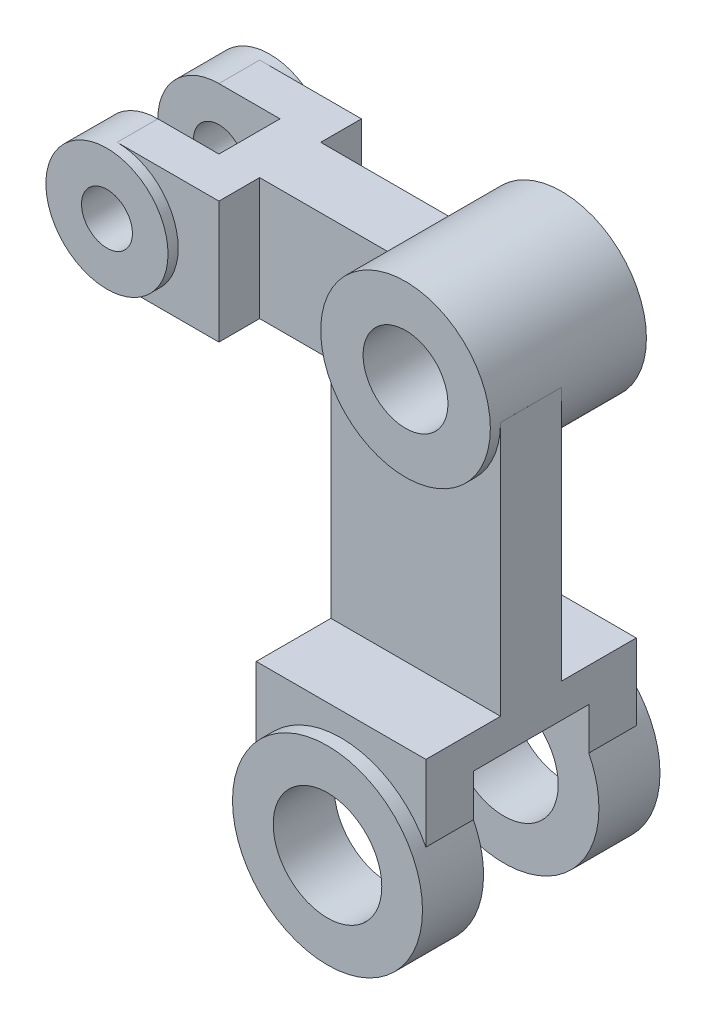
ISO-10303-21;
HEADER;
FILE_DESCRIPTION(('STEP AP214'),'2;1');
FILE_NAME('part.step','',(''),(''),'','','');
FILE_SCHEMA(('AUTOMOTIVE_DESIGN { 1 0 10303 214 1 1 1 1 }'));
ENDSEC;
DATA;
#1=APPLICATION_CONTEXT('core data for automotive mechanical design processes');
#2=APPLICATION_PROTOCOL_DEFINITION('international standard','automotive_design',2000,#1);
#3=PRODUCT_CONTEXT('',#1,'mechanical');
#4=PRODUCT('Part','Part','',(#3));
#5=PRODUCT_RELATED_PRODUCT_CATEGORY('part','',(#4));
#6=PRODUCT_DEFINITION_FORMATION('','',#4);
#7=PRODUCT_DEFINITION_CONTEXT('part definition',#1,'design');
#8=PRODUCT_DEFINITION('design','',#6,#7);
#9=PRODUCT_DEFINITION_SHAPE('','',#8);
#10=(LENGTH_UNIT() NAMED_UNIT(*) SI_UNIT(.MILLI.,.METRE.));
#11=(NAMED_UNIT(*) PLANE_ANGLE_UNIT() SI_UNIT($,.RADIAN.));
#12=(NAMED_UNIT(*) SI_UNIT($,.STERADIAN.) SOLID_ANGLE_UNIT());
#13=UNCERTAINTY_MEASURE_WITH_UNIT(LENGTH_MEASURE(1.E-05),#10,'distance_accuracy_value','');
#14=(GEOMETRIC_REPRESENTATION_CONTEXT(3) GLOBAL_UNCERTAINTY_ASSIGNED_CONTEXT((#13)) GLOBAL_UNIT_ASSIGNED_CONTEXT((#10,
#11,#12)) REPRESENTATION_CONTEXT('',''));
#15=CARTESIAN_POINT('',(0.,0.,0.));
#16=DIRECTION('',(0.,0.,1.));
#17=DIRECTION('',(1.,0.,0.));
#18=AXIS2_PLACEMENT_3D('',#15,#16,#17);
#19=CARTESIAN_POINT('',(0.,110.,0.));
#20=DIRECTION('',(0.,1.,0.));
#21=DIRECTION('',(0.,0.,1.));
#22=AXIS2_PLACEMENT_3D('',#19,#20,#21);
#23=PLANE('',#22);
#24=DIRECTION('',(1.,0.,0.));
#25=VECTOR('',#24,1.);
#26=CARTESIAN_POINT('',(0.,110.,-35.));
#27=LINE('',#26,#25);
#28=CARTESIAN_POINT('',(-25.,110.,-35.));
#29=VERTEX_POINT('',#28);
#30=CARTESIAN_POINT('',(-24.9978511346783,110.,-35.));
#31=VERTEX_POINT('',#30);
#32=EDGE_CURVE('E316',#29,#31,#27,.T.);
#33=ORIENTED_EDGE('',*,*,#32,.F.);
#34=DIRECTION('',(0.,0.,1.));
#35=VECTOR('',#34,1.);
#36=CARTESIAN_POINT('',(-25.,110.,-44.));
#37=LINE('',#36,#35);
#38=CARTESIAN_POINT('',(-25.,110.,-26.));
#39=VERTEX_POINT('',#38);
#40=EDGE_CURVE('E346',#29,#39,#37,.T.);
#41=ORIENTED_EDGE('',*,*,#40,.T.);
#42=DIRECTION('',(1.,0.,0.));
#43=VECTOR('',#42,1.);
#44=CARTESIAN_POINT('',(-25.,110.,-26.));
#45=LINE('',#44,#43);
#46=CARTESIAN_POINT('',(-24.9978511346783,110.,-26.));
#47=VERTEX_POINT('',#46);
#48=EDGE_CURVE('E351',#39,#47,#45,.T.);
#49=ORIENTED_EDGE('',*,*,#48,.T.);
#50=DIRECTION('',(0.,0.,1.));
#51=VECTOR('',#50,1.);
#52=CARTESIAN_POINT('',(-24.9978511346783,110.,-69.));
#53=LINE('',#52,#51);
#54=EDGE_CURVE('E465',#31,#47,#53,.T.);
#55=ORIENTED_EDGE('',*,*,#54,.F.);
#56=EDGE_LOOP('',(#33,#41,#49,#55));
#57=FACE_BOUND('',#56,.T.);
#58=ADVANCED_FACE('F44',(#57),#23,.T.);
#59=CARTESIAN_POINT('',(0.,35.,0.));
#60=DIRECTION('',(0.,-1.,0.));
#61=DIRECTION('',(0.,0.,-1.));
#62=AXIS2_PLACEMENT_3D('',#59,#60,#61);
#63=PLANE('',#62);
#64=DIRECTION('',(-1.,0.,0.));
#65=VECTOR('',#64,1.);
#66=CARTESIAN_POINT('',(-25.,35.,-44.));
#67=LINE('',#66,#65);
#68=CARTESIAN_POINT('',(25.0042977306435,35.,-44.));
#69=VERTEX_POINT('',#68);
#70=CARTESIAN_POINT('',(-25.,35.,-44.));
#71=VERTEX_POINT('',#70);
#72=EDGE_CURVE('E354',#69,#71,#67,.T.);
#73=ORIENTED_EDGE('',*,*,#72,.F.);
#74=DIRECTION('',(0.,0.,-1.));
#75=VECTOR('',#74,1.);
#76=CARTESIAN_POINT('',(25.0042977306435,35.,0.));
#77=LINE('',#76,#75);
#78=CARTESIAN_POINT('',(25.0042977306435,35.,-66.));
#79=VERTEX_POINT('',#78);
#80=EDGE_CURVE('E448',#69,#79,#77,.T.);
#81=ORIENTED_EDGE('',*,*,#80,.T.);
#82=DIRECTION('',(-1.,0.,0.));
#83=VECTOR('',#82,1.);
#84=CARTESIAN_POINT('',(-28.,35.,-66.));
#85=LINE('',#84,#83);
#86=CARTESIAN_POINT('',(-25.,35.,-66.));
#87=VERTEX_POINT('',#86);
#88=EDGE_CURVE('E429',#79,#87,#85,.T.);
#89=ORIENTED_EDGE('',*,*,#88,.T.);
#90=DIRECTION('',(0.,0.,1.));
#91=VECTOR('',#90,1.);
#92=CARTESIAN_POINT('',(-25.,35.,0.));
#93=LINE('',#92,#91);
#94=EDGE_CURVE('E450',#87,#71,#93,.T.);
#95=ORIENTED_EDGE('',*,*,#94,.T.);
#96=EDGE_LOOP('',(#73,#81,#89,#95));
#97=FACE_BOUND('',#96,.T.);
#98=ADVANCED_FACE('F520',(#97),#63,.F.);
#99=DIRECTION('',(1.,0.,0.));
#100=VECTOR('',#99,1.);
#101=CARTESIAN_POINT('',(-25.,35.,-26.));
#102=LINE('',#101,#100);
#103=CARTESIAN_POINT('',(-25.,35.,-26.));
#104=VERTEX_POINT('',#103);
#105=CARTESIAN_POINT('',(25.0042977306435,35.,-26.));
#106=VERTEX_POINT('',#105);
#107=EDGE_CURVE('E350',#104,#106,#102,.T.);
#108=ORIENTED_EDGE('',*,*,#107,.F.);
#109=CARTESIAN_POINT('',(-25.,35.,-4.));
#110=VERTEX_POINT('',#109);
#111=EDGE_CURVE('E447',#104,#110,#93,.T.);
#112=ORIENTED_EDGE('',*,*,#111,.T.);
#113=DIRECTION('',(1.,0.,0.));
#114=VECTOR('',#113,1.);
#115=CARTESIAN_POINT('',(28.,35.,-4.));
#116=LINE('',#115,#114);
#117=CARTESIAN_POINT('',(25.0042977306435,35.,-4.));
#118=VERTEX_POINT('',#117);
#119=EDGE_CURVE('E428',#110,#118,#116,.T.);
#120=ORIENTED_EDGE('',*,*,#119,.T.);
#121=EDGE_CURVE('E452',#118,#106,#77,.T.);
#122=ORIENTED_EDGE('',*,*,#121,.T.);
#123=EDGE_LOOP('',(#108,#112,#120,#122));
#124=FACE_BOUND('',#123,.T.);
#125=ADVANCED_FACE('F527',(#124),#63,.F.);
#126=CARTESIAN_POINT('',(0.,0.,-70.));
#127=DIRECTION('',(0.,0.,1.));
#128=DIRECTION('',(1.,0.,0.));
#129=AXIS2_PLACEMENT_3D('',#126,#127,#128);
#130=CYLINDRICAL_SURFACE('',#129,28.);
#131=CARTESIAN_POINT('',(0.,0.,-70.));
#132=DIRECTION('',(0.,0.,1.));
#133=DIRECTION('',(1.,0.,0.));
#134=AXIS2_PLACEMENT_3D('',#131,#132,#133);
#135=CIRCLE('',#134,28.);
#136=CARTESIAN_POINT('',(28.,0.,-70.));
#137=VERTEX_POINT('',#136);
#138=EDGE_CURVE('E416',#137,#137,#135,.T.);
#139=ORIENTED_EDGE('',*,*,#138,.T.);
#140=EDGE_LOOP('',(#139));
#141=FACE_BOUND('',#140,.T.);
#142=CARTESIAN_POINT('',(0.,0.,-66.));
#143=DIRECTION('',(0.,0.,-1.));
#144=DIRECTION('',(-1.,0.,0.));
#145=AXIS2_PLACEMENT_3D('',#142,#143,#144);
#146=CIRCLE('',#145,28.);
#147=CARTESIAN_POINT('',(-25.,12.6095202129185,-66.));
#148=VERTEX_POINT('',#147);
#149=CARTESIAN_POINT('',(25.0042977306435,12.6009957938782,-66.));
#150=VERTEX_POINT('',#149);
#151=EDGE_CURVE('E422',#148,#150,#146,.T.);
#152=ORIENTED_EDGE('',*,*,#151,.T.);
#153=DIRECTION('',(0.,0.,1.));
#154=VECTOR('',#153,1.);
#155=CARTESIAN_POINT('',(25.0042977306435,12.6009957938782,-70.));
#156=LINE('',#155,#154);
#157=CARTESIAN_POINT('',(25.0042977306435,12.6009957938782,-52.));
#158=VERTEX_POINT('',#157);
#159=EDGE_CURVE('E376',#150,#158,#156,.T.);
#160=ORIENTED_EDGE('',*,*,#159,.T.);
#161=CARTESIAN_POINT('',(0.,0.,-52.));
#162=DIRECTION('',(0.,0.,1.));
#163=DIRECTION('',(1.,0.,0.));
#164=AXIS2_PLACEMENT_3D('',#161,#162,#163);
#165=CIRCLE('',#164,28.);
#166=CARTESIAN_POINT('',(-25.,12.6095202129185,-52.));
#167=VERTEX_POINT('',#166);
#168=EDGE_CURVE('E417',#167,#158,#165,.T.);
#169=ORIENTED_EDGE('',*,*,#168,.F.);
#170=DIRECTION('',(0.,0.,1.));
#171=VECTOR('',#170,1.);
#172=CARTESIAN_POINT('',(-25.,12.6095202129185,-70.));
#173=LINE('',#172,#171);
#174=EDGE_CURVE('E383',#167,#148,#173,.F.);
#175=ORIENTED_EDGE('',*,*,#174,.T.);
#176=EDGE_LOOP('',(#152,#160,#169,#175));
#177=FACE_BOUND('',#176,.T.);
#178=ADVANCED_FACE('F572',(#141,#177),#130,.T.);
#179=CARTESIAN_POINT('',(0.,0.,-18.));
#180=DIRECTION('',(0.,0.,1.));
#181=DIRECTION('',(1.,0.,0.));
#182=AXIS2_PLACEMENT_3D('',#179,#180,#181);
#183=CYLINDRICAL_SURFACE('',#182,28.);
#184=CARTESIAN_POINT('',(0.,0.,0.));
#185=DIRECTION('',(0.,0.,1.));
#186=DIRECTION('',(1.,0.,0.));
#187=AXIS2_PLACEMENT_3D('',#184,#185,#186);
#188=CIRCLE('',#187,28.);
#189=CARTESIAN_POINT('',(28.,0.,0.));
#190=VERTEX_POINT('',#189);
#191=EDGE_CURVE('E436',#190,#190,#188,.T.);
#192=ORIENTED_EDGE('',*,*,#191,.F.);
#193=EDGE_LOOP('',(#192));
#194=FACE_BOUND('',#193,.T.);
#195=CARTESIAN_POINT('',(0.,0.,-18.));
#196=DIRECTION('',(0.,0.,1.));
#197=DIRECTION('',(1.,0.,0.));
#198=AXIS2_PLACEMENT_3D('',#195,#196,#197);
#199=CIRCLE('',#198,28.);
#200=CARTESIAN_POINT('',(-25.,12.6095202129185,-18.));
#201=VERTEX_POINT('',#200);
#202=CARTESIAN_POINT('',(25.0042977306435,12.6009957938782,-18.));
#203=VERTEX_POINT('',#202);
#204=EDGE_CURVE('E437',#201,#203,#199,.T.);
#205=ORIENTED_EDGE('',*,*,#204,.T.);
#206=DIRECTION('',(0.,0.,1.));
#207=VECTOR('',#206,1.);
#208=CARTESIAN_POINT('',(25.0042977306435,12.6009957938782,-18.));
#209=LINE('',#208,#207);
#210=CARTESIAN_POINT('',(25.0042977306435,12.6009957938782,-4.));
#211=VERTEX_POINT('',#210);
#212=EDGE_CURVE('E378',#203,#211,#209,.T.);
#213=ORIENTED_EDGE('',*,*,#212,.T.);
#214=CARTESIAN_POINT('',(0.,0.,-4.));
#215=DIRECTION('',(0.,0.,1.));
#216=DIRECTION('',(1.,0.,0.));
#217=AXIS2_PLACEMENT_3D('',#214,#215,#216);
#218=CIRCLE('',#217,28.);
#219=CARTESIAN_POINT('',(-25.,12.6095202129185,-4.));
#220=VERTEX_POINT('',#219);
#221=EDGE_CURVE('E445',#220,#211,#218,.F.);
#222=ORIENTED_EDGE('',*,*,#221,.F.);
#223=DIRECTION('',(0.,0.,1.));
#224=VECTOR('',#223,1.);
#225=CARTESIAN_POINT('',(-25.,12.6095202129185,-18.));
#226=LINE('',#225,#224);
#227=EDGE_CURVE('E385',#220,#201,#226,.F.);
#228=ORIENTED_EDGE('',*,*,#227,.T.);
#229=EDGE_LOOP('',(#205,#213,#222,#228));
#230=FACE_BOUND('',#229,.T.);
#231=ADVANCED_FACE('F50',(#194,#230),#183,.T.);
#232=CARTESIAN_POINT('',(0.,0.,-18.));
#233=DIRECTION('',(0.,0.,1.));
#234=DIRECTION('',(1.,0.,0.));
#235=AXIS2_PLACEMENT_3D('',#232,#233,#234);
#236=PLANE('',#235);
#237=DIRECTION('',(0.,1.,0.));
#238=VECTOR('',#237,1.);
#239=CARTESIAN_POINT('',(25.0042977306435,17.,-18.));
#240=LINE('',#239,#238);
#241=CARTESIAN_POINT('',(25.0042977306435,25.,-18.));
#242=VERTEX_POINT('',#241);
#243=EDGE_CURVE('E454',#203,#242,#240,.T.);
#244=ORIENTED_EDGE('',*,*,#243,.F.);
#245=ORIENTED_EDGE('',*,*,#204,.F.);
#246=DIRECTION('',(0.,1.,0.));
#247=VECTOR('',#246,1.);
#248=CARTESIAN_POINT('',(-25.,17.,-18.));
#249=LINE('',#248,#247);
#250=CARTESIAN_POINT('',(-25.,25.,-18.));
#251=VERTEX_POINT('',#250);
#252=EDGE_CURVE('E388',#201,#251,#249,.T.);
#253=ORIENTED_EDGE('',*,*,#252,.T.);
#254=DIRECTION('',(-1.,0.,0.));
#255=VECTOR('',#254,1.);
#256=CARTESIAN_POINT('',(28.,25.,-18.));
#257=LINE('',#256,#255);
#258=EDGE_CURVE('E397',#242,#251,#257,.T.);
#259=ORIENTED_EDGE('',*,*,#258,.F.);
#260=EDGE_LOOP('',(#244,#245,#253,#259));
#261=FACE_BOUND('',#260,.T.);
#262=CARTESIAN_POINT('',(0.,0.,-18.));
#263=DIRECTION('',(0.,0.,1.));
#264=DIRECTION('',(1.,0.,0.));
#265=AXIS2_PLACEMENT_3D('',#262,#263,#264);
#266=CIRCLE('',#265,16.);
#267=CARTESIAN_POINT('',(16.,0.,-18.));
#268=VERTEX_POINT('',#267);
#269=EDGE_CURVE('E433',#268,#268,#266,.T.);
#270=ORIENTED_EDGE('',*,*,#269,.T.);
#271=EDGE_LOOP('',(#270));
#272=FACE_BOUND('',#271,.T.);
#273=ADVANCED_FACE('F590',(#261,#272),#236,.F.);
#274=CARTESIAN_POINT('',(0.,0.,0.));
#275=DIRECTION('',(0.,0.,1.));
#276=DIRECTION('',(1.,0.,0.));
#277=AXIS2_PLACEMENT_3D('',#274,#275,#276);
#278=PLANE('',#277);
#279=CARTESIAN_POINT('',(0.,0.,0.));
#280=DIRECTION('',(0.,0.,1.));
#281=DIRECTION('',(1.,0.,0.));
#282=AXIS2_PLACEMENT_3D('',#279,#280,#281);
#283=CIRCLE('',#282,16.);
#284=CARTESIAN_POINT('',(16.,0.,0.));
#285=VERTEX_POINT('',#284);
#286=EDGE_CURVE('E435',#285,#285,#283,.T.);
#287=ORIENTED_EDGE('',*,*,#286,.F.);
#288=EDGE_LOOP('',(#287));
#289=FACE_BOUND('',#288,.T.);
#290=ORIENTED_EDGE('',*,*,#191,.T.);
#291=EDGE_LOOP('',(#290));
#292=FACE_BOUND('',#291,.T.);
#293=ADVANCED_FACE('F589',(#289,#292),#278,.T.);
#294=CARTESIAN_POINT('',(0.,0.,-18.));
#295=DIRECTION('',(0.,0.,1.));
#296=DIRECTION('',(1.,0.,0.));
#297=AXIS2_PLACEMENT_3D('',#294,#295,#296);
#298=CYLINDRICAL_SURFACE('',#297,16.);
#299=ORIENTED_EDGE('',*,*,#269,.F.);
#300=EDGE_LOOP('',(#299));
#301=FACE_BOUND('',#300,.T.);
#302=ORIENTED_EDGE('',*,*,#286,.T.);
#303=EDGE_LOOP('',(#302));
#304=FACE_BOUND('',#303,.T.);
#305=ADVANCED_FACE('F578',(#301,#304),#298,.F.);
#306=CARTESIAN_POINT('',(-28.,17.,-66.));
#307=DIRECTION('',(0.,0.,-1.));
#308=DIRECTION('',(-1.,0.,0.));
#309=AXIS2_PLACEMENT_3D('',#306,#307,#308);
#310=PLANE('',#309);
#311=DIRECTION('',(0.,1.,0.));
#312=VECTOR('',#311,1.);
#313=CARTESIAN_POINT('',(25.0042977306435,17.,-66.));
#314=LINE('',#313,#312);
#315=EDGE_CURVE('E406',#150,#79,#314,.T.);
#316=ORIENTED_EDGE('',*,*,#315,.F.);
#317=ORIENTED_EDGE('',*,*,#151,.F.);
#318=DIRECTION('',(0.,-1.,0.));
#319=VECTOR('',#318,1.);
#320=CARTESIAN_POINT('',(-25.,17.,-66.));
#321=LINE('',#320,#319);
#322=EDGE_CURVE('E404',#87,#148,#321,.T.);
#323=ORIENTED_EDGE('',*,*,#322,.F.);
#324=ORIENTED_EDGE('',*,*,#88,.F.);
#325=EDGE_LOOP('',(#316,#317,#323,#324));
#326=FACE_BOUND('',#325,.T.);
#327=ADVANCED_FACE('F580',(#326),#310,.T.);
#328=CARTESIAN_POINT('',(28.,17.,-4.));
#329=DIRECTION('',(0.,0.,1.));
#330=DIRECTION('',(1.,0.,0.));
#331=AXIS2_PLACEMENT_3D('',#328,#329,#330);
#332=PLANE('',#331);
#333=DIRECTION('',(0.,-1.,0.));
#334=VECTOR('',#333,1.);
#335=CARTESIAN_POINT('',(25.0042977306435,17.,-4.));
#336=LINE('',#335,#334);
#337=EDGE_CURVE('E402',#118,#211,#336,.T.);
#338=ORIENTED_EDGE('',*,*,#337,.F.);
#339=ORIENTED_EDGE('',*,*,#119,.F.);
#340=DIRECTION('',(0.,1.,0.));
#341=VECTOR('',#340,1.);
#342=CARTESIAN_POINT('',(-25.,17.,-4.));
#343=LINE('',#342,#341);
#344=EDGE_CURVE('E396',#220,#110,#343,.T.);
#345=ORIENTED_EDGE('',*,*,#344,.F.);
#346=ORIENTED_EDGE('',*,*,#221,.T.);
#347=EDGE_LOOP('',(#338,#339,#345,#346));
#348=FACE_BOUND('',#347,.T.);
#349=ADVANCED_FACE('F568',(#348),#332,.T.);
#350=CARTESIAN_POINT('',(0.,0.,-70.));
#351=DIRECTION('',(0.,0.,1.));
#352=DIRECTION('',(1.,0.,0.));
#353=AXIS2_PLACEMENT_3D('',#350,#351,#352);
#354=PLANE('',#353);
#355=CARTESIAN_POINT('',(0.,0.,-70.));
#356=DIRECTION('',(0.,0.,1.));
#357=DIRECTION('',(1.,0.,0.));
#358=AXIS2_PLACEMENT_3D('',#355,#356,#357);
#359=CIRCLE('',#358,16.);
#360=CARTESIAN_POINT('',(16.,0.,-70.));
#361=VERTEX_POINT('',#360);
#362=EDGE_CURVE('E412',#361,#361,#359,.T.);
#363=ORIENTED_EDGE('',*,*,#362,.T.);
#364=EDGE_LOOP('',(#363));
#365=FACE_BOUND('',#364,.T.);
#366=ORIENTED_EDGE('',*,*,#138,.F.);
#367=EDGE_LOOP('',(#366));
#368=FACE_BOUND('',#367,.T.);
#369=ADVANCED_FACE('F564',(#365,#368),#354,.F.);
#370=CARTESIAN_POINT('',(0.,0.,-52.));
#371=DIRECTION('',(0.,0.,1.));
#372=DIRECTION('',(1.,0.,0.));
#373=AXIS2_PLACEMENT_3D('',#370,#371,#372);
#374=PLANE('',#373);
#375=ORIENTED_EDGE('',*,*,#168,.T.);
#376=DIRECTION('',(0.,-1.,0.));
#377=VECTOR('',#376,1.);
#378=CARTESIAN_POINT('',(25.0042977306435,17.,-52.));
#379=LINE('',#378,#377);
#380=CARTESIAN_POINT('',(25.0042977306435,25.,-52.));
#381=VERTEX_POINT('',#380);
#382=EDGE_CURVE('E460',#381,#158,#379,.T.);
#383=ORIENTED_EDGE('',*,*,#382,.F.);
#384=DIRECTION('',(-1.,0.,0.));
#385=VECTOR('',#384,1.);
#386=CARTESIAN_POINT('',(28.,25.,-52.));
#387=LINE('',#386,#385);
#388=CARTESIAN_POINT('',(-25.,25.,-52.));
#389=VERTEX_POINT('',#388);
#390=EDGE_CURVE('E400',#381,#389,#387,.T.);
#391=ORIENTED_EDGE('',*,*,#390,.T.);
#392=DIRECTION('',(0.,-1.,0.));
#393=VECTOR('',#392,1.);
#394=CARTESIAN_POINT('',(-25.,17.,-52.));
#395=LINE('',#394,#393);
#396=EDGE_CURVE('E389',#389,#167,#395,.T.);
#397=ORIENTED_EDGE('',*,*,#396,.T.);
#398=EDGE_LOOP('',(#375,#383,#391,#397));
#399=FACE_BOUND('',#398,.T.);
#400=CARTESIAN_POINT('',(0.,0.,-52.));
#401=DIRECTION('',(0.,0.,1.));
#402=DIRECTION('',(1.,0.,0.));
#403=AXIS2_PLACEMENT_3D('',#400,#401,#402);
#404=CIRCLE('',#403,16.);
#405=CARTESIAN_POINT('',(16.,0.,-52.));
#406=VERTEX_POINT('',#405);
#407=EDGE_CURVE('E414',#406,#406,#404,.T.);
#408=ORIENTED_EDGE('',*,*,#407,.F.);
#409=EDGE_LOOP('',(#408));
#410=FACE_BOUND('',#409,.T.);
#411=ADVANCED_FACE('F563',(#399,#410),#374,.T.);
#412=CARTESIAN_POINT('',(0.,0.,-70.));
#413=DIRECTION('',(0.,0.,1.));
#414=DIRECTION('',(1.,0.,0.));
#415=AXIS2_PLACEMENT_3D('',#412,#413,#414);
#416=CYLINDRICAL_SURFACE('',#415,16.);
#417=ORIENTED_EDGE('',*,*,#362,.F.);
#418=EDGE_LOOP('',(#417));
#419=FACE_BOUND('',#418,.T.);
#420=ORIENTED_EDGE('',*,*,#407,.T.);
#421=EDGE_LOOP('',(#420));
#422=FACE_BOUND('',#421,.T.);
#423=ADVANCED_FACE('F559',(#419,#422),#416,.F.);
#424=CARTESIAN_POINT('',(-25.,17.,-70.));
#425=DIRECTION('',(1.,0.,0.));
#426=DIRECTION('',(0.,0.,-1.));
#427=AXIS2_PLACEMENT_3D('',#424,#425,#426);
#428=PLANE('',#427);
#429=ORIENTED_EDGE('',*,*,#40,.F.);
#430=DIRECTION('',(0.,-1.,0.));
#431=VECTOR('',#430,1.);
#432=CARTESIAN_POINT('',(-25.,17.,-35.));
#433=LINE('',#432,#431);
#434=CARTESIAN_POINT('',(-25.,92.,-35.));
#435=VERTEX_POINT('',#434);
#436=EDGE_CURVE('E322',#29,#435,#433,.T.);
#437=ORIENTED_EDGE('',*,*,#436,.T.);
#438=DIRECTION('',(0.,0.,-1.));
#439=VECTOR('',#438,1.);
#440=CARTESIAN_POINT('',(-25.,92.,-70.));
#441=LINE('',#440,#439);
#442=CARTESIAN_POINT('',(-25.,92.,-44.));
#443=VERTEX_POINT('',#442);
#444=EDGE_CURVE('E330',#435,#443,#441,.T.);
#445=ORIENTED_EDGE('',*,*,#444,.T.);
#446=DIRECTION('',(0.,-1.,0.));
#447=VECTOR('',#446,1.);
#448=CARTESIAN_POINT('',(-25.,110.,-44.));
#449=LINE('',#448,#447);
#450=EDGE_CURVE('E363',#443,#71,#449,.T.);
#451=ORIENTED_EDGE('',*,*,#450,.T.);
#452=ORIENTED_EDGE('',*,*,#94,.F.);
#453=ORIENTED_EDGE('',*,*,#322,.T.);
#454=ORIENTED_EDGE('',*,*,#174,.F.);
#455=ORIENTED_EDGE('',*,*,#396,.F.);
#456=DIRECTION('',(0.,0.,-1.));
#457=VECTOR('',#456,1.);
#458=CARTESIAN_POINT('',(-25.,25.,-52.));
#459=LINE('',#458,#457);
#460=EDGE_CURVE('E392',#251,#389,#459,.T.);
#461=ORIENTED_EDGE('',*,*,#460,.F.);
#462=ORIENTED_EDGE('',*,*,#252,.F.);
#463=ORIENTED_EDGE('',*,*,#227,.F.);
#464=ORIENTED_EDGE('',*,*,#344,.T.);
#465=ORIENTED_EDGE('',*,*,#111,.F.);
#466=DIRECTION('',(0.,-1.,0.));
#467=VECTOR('',#466,1.);
#468=CARTESIAN_POINT('',(-25.,110.,-26.));
#469=LINE('',#468,#467);
#470=EDGE_CURVE('E373',#39,#104,#469,.T.);
#471=ORIENTED_EDGE('',*,*,#470,.F.);
#472=EDGE_LOOP('',(#429,#437,#445,#451,#452,#453,#454,#455,#461,#462,#463,#464,#465,#471));
#473=FACE_BOUND('',#472,.T.);
#474=ADVANCED_FACE('F558',(#473),#428,.F.);
#475=CARTESIAN_POINT('',(25.0042977306435,17.,-70.));
#476=DIRECTION('',(-1.,0.,0.));
#477=DIRECTION('',(0.,-1.,0.));
#478=AXIS2_PLACEMENT_3D('',#475,#476,#477);
#479=PLANE('',#478);
#480=DIRECTION('',(0.,0.,-1.));
#481=VECTOR('',#480,1.);
#482=CARTESIAN_POINT('',(25.0042977306435,25.,-70.));
#483=LINE('',#482,#481);
#484=EDGE_CURVE('E458',#242,#381,#483,.T.);
#485=ORIENTED_EDGE('',*,*,#484,.T.);
#486=ORIENTED_EDGE('',*,*,#382,.T.);
#487=ORIENTED_EDGE('',*,*,#159,.F.);
#488=ORIENTED_EDGE('',*,*,#315,.T.);
#489=ORIENTED_EDGE('',*,*,#80,.F.);
#490=DIRECTION('',(0.,-1.,0.));
#491=VECTOR('',#490,1.);
#492=CARTESIAN_POINT('',(25.0042977306435,110.,-44.));
#493=LINE('',#492,#491);
#494=CARTESIAN_POINT('',(25.0042977306435,110.,-44.));
#495=VERTEX_POINT('',#494);
#496=EDGE_CURVE('E370',#495,#69,#493,.T.);
#497=ORIENTED_EDGE('',*,*,#496,.F.);
#498=DIRECTION('',(0.,0.,-1.));
#499=VECTOR('',#498,1.);
#500=CARTESIAN_POINT('',(25.0042977306435,110.,-44.));
#501=LINE('',#500,#499);
#502=CARTESIAN_POINT('',(25.0042977306435,110.,-26.));
#503=VERTEX_POINT('',#502);
#504=EDGE_CURVE('E357',#503,#495,#501,.T.);
#505=ORIENTED_EDGE('',*,*,#504,.F.);
#506=DIRECTION('',(0.,-1.,0.));
#507=VECTOR('',#506,1.);
#508=CARTESIAN_POINT('',(25.0042977306435,110.,-26.));
#509=LINE('',#508,#507);
#510=EDGE_CURVE('E369',#503,#106,#509,.T.);
#511=ORIENTED_EDGE('',*,*,#510,.T.);
#512=ORIENTED_EDGE('',*,*,#121,.F.);
#513=ORIENTED_EDGE('',*,*,#337,.T.);
#514=ORIENTED_EDGE('',*,*,#212,.F.);
#515=ORIENTED_EDGE('',*,*,#243,.T.);
#516=EDGE_LOOP('',(#485,#486,#487,#488,#489,#497,#505,#511,#512,#513,#514,#515));
#517=FACE_BOUND('',#516,.T.);
#518=ADVANCED_FACE('F552',(#517),#479,.F.);
#519=CARTESIAN_POINT('',(28.,25.,-52.));
#520=DIRECTION('',(0.,1.,0.));
#521=DIRECTION('',(0.,0.,1.));
#522=AXIS2_PLACEMENT_3D('',#519,#520,#521);
#523=PLANE('',#522);
#524=ORIENTED_EDGE('',*,*,#258,.T.);
#525=ORIENTED_EDGE('',*,*,#460,.T.);
#526=ORIENTED_EDGE('',*,*,#390,.F.);
#527=ORIENTED_EDGE('',*,*,#484,.F.);
#528=EDGE_LOOP('',(#524,#525,#526,#527));
#529=FACE_BOUND('',#528,.T.);
#530=ADVANCED_FACE('F541',(#529),#523,.F.);
#531=CARTESIAN_POINT('',(-25.,110.,-26.));
#532=DIRECTION('',(0.,0.,-1.));
#533=DIRECTION('',(-1.,0.,0.));
#534=AXIS2_PLACEMENT_3D('',#531,#532,#533);
#535=PLANE('',#534);
#536=CARTESIAN_POINT('',(25.0021488653217,110.,-26.));
#537=VERTEX_POINT('',#536);
#538=EDGE_CURVE('E355',#537,#503,#45,.T.);
#539=ORIENTED_EDGE('',*,*,#538,.F.);
#540=CARTESIAN_POINT('',(0.00214886532174871,110.,-26.));
#541=DIRECTION('',(0.,0.,-1.));
#542=DIRECTION('',(-1.,0.,0.));
#543=AXIS2_PLACEMENT_3D('',#540,#541,#542);
#544=CIRCLE('',#543,25.);
#545=EDGE_CURVE('E348',#537,#47,#544,.T.);
#546=ORIENTED_EDGE('',*,*,#545,.T.);
#547=ORIENTED_EDGE('',*,*,#48,.F.);
#548=ORIENTED_EDGE('',*,*,#470,.T.);
#549=ORIENTED_EDGE('',*,*,#107,.T.);
#550=ORIENTED_EDGE('',*,*,#510,.F.);
#551=EDGE_LOOP('',(#539,#546,#547,#548,#549,#550));
#552=FACE_BOUND('',#551,.T.);
#553=ADVANCED_FACE('F543',(#552),#535,.F.);
#554=CARTESIAN_POINT('',(-25.,110.,-44.));
#555=DIRECTION('',(0.,0.,1.));
#556=DIRECTION('',(1.,0.,0.));
#557=AXIS2_PLACEMENT_3D('',#554,#555,#556);
#558=PLANE('',#557);
#559=ORIENTED_EDGE('',*,*,#450,.F.);
#560=DIRECTION('',(1.,0.,0.));
#561=VECTOR('',#560,1.);
#562=CARTESIAN_POINT('',(-25.,92.,-44.));
#563=LINE('',#562,#561);
#564=CARTESIAN_POINT('',(-17.3472027075757,92.,-44.));
#565=VERTEX_POINT('',#564);
#566=EDGE_CURVE('E328',#443,#565,#563,.T.);
#567=ORIENTED_EDGE('',*,*,#566,.T.);
#568=CARTESIAN_POINT('',(0.00214886532174871,110.,-44.));
#569=DIRECTION('',(0.,0.,1.));
#570=DIRECTION('',(1.,0.,0.));
#571=AXIS2_PLACEMENT_3D('',#568,#569,#570);
#572=CIRCLE('',#571,25.);
#573=CARTESIAN_POINT('',(25.0021488653218,110.,-44.));
#574=VERTEX_POINT('',#573);
#575=EDGE_CURVE('E345',#565,#574,#572,.T.);
#576=ORIENTED_EDGE('',*,*,#575,.T.);
#577=DIRECTION('',(-1.,0.,0.));
#578=VECTOR('',#577,1.);
#579=CARTESIAN_POINT('',(-25.,110.,-44.));
#580=LINE('',#579,#578);
#581=EDGE_CURVE('E360',#495,#574,#580,.T.);
#582=ORIENTED_EDGE('',*,*,#581,.F.);
#583=ORIENTED_EDGE('',*,*,#496,.T.);
#584=ORIENTED_EDGE('',*,*,#72,.T.);
#585=EDGE_LOOP('',(#559,#567,#576,#582,#583,#584));
#586=FACE_BOUND('',#585,.T.);
#587=ADVANCED_FACE('F531',(#586),#558,.F.);
#588=DIRECTION('',(0.,0.,1.));
#589=VECTOR('',#588,1.);
#590=CARTESIAN_POINT('',(25.0021488653218,110.,-69.));
#591=LINE('',#590,#589);
#592=EDGE_CURVE('E67',#537,#574,#591,.F.);
#593=ORIENTED_EDGE('',*,*,#592,.F.);
#594=ORIENTED_EDGE('',*,*,#538,.T.);
#595=ORIENTED_EDGE('',*,*,#504,.T.);
#596=ORIENTED_EDGE('',*,*,#581,.T.);
#597=EDGE_LOOP('',(#593,#594,#595,#596));
#598=FACE_BOUND('',#597,.T.);
#599=ADVANCED_FACE('F518',(#598),#23,.T.);
#600=CARTESIAN_POINT('',(0.00214886532174871,110.,-69.));
#601=DIRECTION('',(0.,0.,1.));
#602=DIRECTION('',(1.,0.,0.));
#603=AXIS2_PLACEMENT_3D('',#600,#601,#602);
#604=CYLINDRICAL_SURFACE('',#603,25.);
#605=DIRECTION('',(0.,0.,1.));
#606=VECTOR('',#605,1.);
#607=CARTESIAN_POINT('',(-17.3472027075757,92.,-69.));
#608=LINE('',#607,#606);
#609=CARTESIAN_POINT('',(-17.3472027075757,92.,-53.));
#610=VERTEX_POINT('',#609);
#611=EDGE_CURVE('E11',#610,#565,#608,.T.);
#612=ORIENTED_EDGE('',*,*,#611,.F.);
#613=CARTESIAN_POINT('',(0.00214886532174871,110.,-53.));
#614=DIRECTION('',(0.,0.,-1.));
#615=DIRECTION('',(-1.,0.,0.));
#616=AXIS2_PLACEMENT_3D('',#613,#614,#615);
#617=CIRCLE('',#616,25.);
#618=CARTESIAN_POINT('',(-17.3472027075757,128.,-53.));
#619=VERTEX_POINT('',#618);
#620=EDGE_CURVE('E321',#619,#610,#617,.F.);
#621=ORIENTED_EDGE('',*,*,#620,.F.);
#622=DIRECTION('',(0.,0.,1.));
#623=VECTOR('',#622,1.);
#624=CARTESIAN_POINT('',(-17.3472027075757,128.,-69.));
#625=LINE('',#624,#623);
#626=CARTESIAN_POINT('',(-17.3472027075757,128.,-35.));
#627=VERTEX_POINT('',#626);
#628=EDGE_CURVE('E52',#619,#627,#625,.T.);
#629=ORIENTED_EDGE('',*,*,#628,.T.);
#630=CARTESIAN_POINT('',(0.00214886532174871,110.,-35.));
#631=DIRECTION('',(0.,0.,1.));
#632=DIRECTION('',(1.,0.,0.));
#633=AXIS2_PLACEMENT_3D('',#630,#631,#632);
#634=CIRCLE('',#633,25.);
#635=EDGE_CURVE('E310',#31,#627,#634,.F.);
#636=ORIENTED_EDGE('',*,*,#635,.F.);
#637=ORIENTED_EDGE('',*,*,#54,.T.);
#638=ORIENTED_EDGE('',*,*,#545,.F.);
#639=ORIENTED_EDGE('',*,*,#592,.T.);
#640=ORIENTED_EDGE('',*,*,#575,.F.);
#641=EDGE_LOOP('',(#612,#621,#629,#636,#637,#638,#639,#640));
#642=FACE_BOUND('',#641,.T.);
#643=CARTESIAN_POINT('',(0.00214886532174871,110.,-69.));
#644=DIRECTION('',(0.,0.,1.));
#645=DIRECTION('',(1.,0.,0.));
#646=AXIS2_PLACEMENT_3D('',#643,#644,#645);
#647=CIRCLE('',#646,25.);
#648=CARTESIAN_POINT('',(25.0021488653218,110.,-69.));
#649=VERTEX_POINT('',#648);
#650=EDGE_CURVE('E339',#649,#649,#647,.T.);
#651=ORIENTED_EDGE('',*,*,#650,.T.);
#652=EDGE_LOOP('',(#651));
#653=FACE_BOUND('',#652,.T.);
#654=CARTESIAN_POINT('',(0.00214886532174871,110.,-23.));
#655=DIRECTION('',(0.,0.,1.));
#656=DIRECTION('',(1.,0.,0.));
#657=AXIS2_PLACEMENT_3D('',#654,#655,#656);
#658=CIRCLE('',#657,25.);
#659=CARTESIAN_POINT('',(25.0021488653218,110.,-23.));
#660=VERTEX_POINT('',#659);
#661=EDGE_CURVE('E337',#660,#660,#658,.T.);
#662=ORIENTED_EDGE('',*,*,#661,.F.);
#663=EDGE_LOOP('',(#662));
#664=FACE_BOUND('',#663,.T.);
#665=ADVANCED_FACE('F466',(#642,#653,#664),#604,.T.);
#666=CARTESIAN_POINT('',(0.00214886532174871,110.,-69.));
#667=DIRECTION('',(0.,0.,1.));
#668=DIRECTION('',(1.,0.,0.));
#669=AXIS2_PLACEMENT_3D('',#666,#667,#668);
#670=PLANE('',#669);
#671=CARTESIAN_POINT('',(0.00214886532174871,110.,-69.));
#672=DIRECTION('',(0.,0.,1.));
#673=DIRECTION('',(1.,0.,0.));
#674=AXIS2_PLACEMENT_3D('',#671,#672,#673);
#675=CIRCLE('',#674,12.5);
#676=CARTESIAN_POINT('',(12.5021488653217,110.,-69.));
#677=VERTEX_POINT('',#676);
#678=EDGE_CURVE('E334',#677,#677,#675,.T.);
#679=ORIENTED_EDGE('',*,*,#678,.T.);
#680=EDGE_LOOP('',(#679));
#681=FACE_BOUND('',#680,.T.);
#682=ORIENTED_EDGE('',*,*,#650,.F.);
#683=EDGE_LOOP('',(#682));
#684=FACE_BOUND('',#683,.T.);
#685=ADVANCED_FACE('F536',(#681,#684),#670,.F.);
#686=CARTESIAN_POINT('',(0.00214886532174871,110.,-23.));
#687=DIRECTION('',(0.,0.,1.));
#688=DIRECTION('',(1.,0.,0.));
#689=AXIS2_PLACEMENT_3D('',#686,#687,#688);
#690=PLANE('',#689);
#691=CARTESIAN_POINT('',(0.00214886532174871,110.,-23.));
#692=DIRECTION('',(0.,0.,1.));
#693=DIRECTION('',(1.,0.,0.));
#694=AXIS2_PLACEMENT_3D('',#691,#692,#693);
#695=CIRCLE('',#694,12.5);
#696=CARTESIAN_POINT('',(12.5021488653217,110.,-23.));
#697=VERTEX_POINT('',#696);
#698=EDGE_CURVE('E335',#697,#697,#695,.T.);
#699=ORIENTED_EDGE('',*,*,#698,.F.);
#700=EDGE_LOOP('',(#699));
#701=FACE_BOUND('',#700,.T.);
#702=ORIENTED_EDGE('',*,*,#661,.T.);
#703=EDGE_LOOP('',(#702));
#704=FACE_BOUND('',#703,.T.);
#705=ADVANCED_FACE('F669',(#701,#704),#690,.T.);
#706=CARTESIAN_POINT('',(0.00214886532174871,110.,-69.));
#707=DIRECTION('',(0.,0.,1.));
#708=DIRECTION('',(1.,0.,0.));
#709=AXIS2_PLACEMENT_3D('',#706,#707,#708);
#710=CYLINDRICAL_SURFACE('',#709,12.5);
#711=ORIENTED_EDGE('',*,*,#698,.T.);
#712=EDGE_LOOP('',(#711));
#713=FACE_BOUND('',#712,.T.);
#714=ORIENTED_EDGE('',*,*,#678,.F.);
#715=EDGE_LOOP('',(#714));
#716=FACE_BOUND('',#715,.T.);
#717=ADVANCED_FACE('F663',(#713,#716),#710,.F.);
#718=CARTESIAN_POINT('',(0.,92.,0.));
#719=DIRECTION('',(0.,-1.,0.));
#720=DIRECTION('',(0.,0.,-1.));
#721=AXIS2_PLACEMENT_3D('',#718,#719,#720);
#722=PLANE('',#721);
#723=ORIENTED_EDGE('',*,*,#444,.F.);
#724=DIRECTION('',(1.,0.,0.));
#725=VECTOR('',#724,1.);
#726=CARTESIAN_POINT('',(-4.74570857755996,92.,-35.));
#727=LINE('',#726,#725);
#728=CARTESIAN_POINT('',(-54.9978511346783,92.,-35.));
#729=VERTEX_POINT('',#728);
#730=EDGE_CURVE('E271',#729,#435,#727,.T.);
#731=ORIENTED_EDGE('',*,*,#730,.F.);
#732=DIRECTION('',(0.,0.,-1.));
#733=VECTOR('',#732,1.);
#734=CARTESIAN_POINT('',(-54.9978511346783,92.,-35.));
#735=LINE('',#734,#733);
#736=CARTESIAN_POINT('',(-54.9978511346783,92.,-23.));
#737=VERTEX_POINT('',#736);
#738=EDGE_CURVE('E268',#737,#729,#735,.T.);
#739=ORIENTED_EDGE('',*,*,#738,.F.);
#740=DIRECTION('',(1.,0.,0.));
#741=VECTOR('',#740,1.);
#742=CARTESIAN_POINT('',(-54.9978511346783,92.,-23.));
#743=LINE('',#742,#741);
#744=CARTESIAN_POINT('',(-84.9978511346783,92.,-23.));
#745=VERTEX_POINT('',#744);
#746=EDGE_CURVE('E270',#745,#737,#743,.T.);
#747=ORIENTED_EDGE('',*,*,#746,.F.);
#748=DIRECTION('',(0.,0.,1.));
#749=VECTOR('',#748,1.);
#750=CARTESIAN_POINT('',(-84.9978511346783,92.,-23.));
#751=LINE('',#750,#749);
#752=CARTESIAN_POINT('',(-84.9978511346783,92.,-35.));
#753=VERTEX_POINT('',#752);
#754=EDGE_CURVE('E261',#753,#745,#751,.T.);
#755=ORIENTED_EDGE('',*,*,#754,.F.);
#756=DIRECTION('',(-1.,0.,0.));
#757=VECTOR('',#756,1.);
#758=CARTESIAN_POINT('',(-84.9978511346783,92.,-35.));
#759=LINE('',#758,#757);
#760=CARTESIAN_POINT('',(-66.9978511346783,92.,-35.));
#761=VERTEX_POINT('',#760);
#762=EDGE_CURVE('E253',#761,#753,#759,.T.);
#763=ORIENTED_EDGE('',*,*,#762,.F.);
#764=DIRECTION('',(0.,0.,1.));
#765=VECTOR('',#764,1.);
#766=CARTESIAN_POINT('',(-66.9978511346783,92.,-35.));
#767=LINE('',#766,#765);
#768=CARTESIAN_POINT('',(-66.9978511346783,92.,-53.));
#769=VERTEX_POINT('',#768);
#770=EDGE_CURVE('E255',#769,#761,#767,.T.);
#771=ORIENTED_EDGE('',*,*,#770,.F.);
#772=DIRECTION('',(1.,0.,0.));
#773=VECTOR('',#772,1.);
#774=CARTESIAN_POINT('',(-66.9978511346783,92.,-53.));
#775=LINE('',#774,#773);
#776=CARTESIAN_POINT('',(-84.9978511346783,92.,-53.));
#777=VERTEX_POINT('',#776);
#778=EDGE_CURVE('E241',#777,#769,#775,.T.);
#779=ORIENTED_EDGE('',*,*,#778,.F.);
#780=DIRECTION('',(0.,0.,1.));
#781=VECTOR('',#780,1.);
#782=CARTESIAN_POINT('',(-84.9978511346783,92.,-53.));
#783=LINE('',#782,#781);
#784=CARTESIAN_POINT('',(-84.9978511346783,92.,-65.));
#785=VERTEX_POINT('',#784);
#786=EDGE_CURVE('E221',#785,#777,#783,.T.);
#787=ORIENTED_EDGE('',*,*,#786,.F.);
#788=DIRECTION('',(-1.,0.,0.));
#789=VECTOR('',#788,1.);
#790=CARTESIAN_POINT('',(-84.9978511346783,92.,-65.));
#791=LINE('',#790,#789);
#792=CARTESIAN_POINT('',(-54.9978511346783,92.,-65.));
#793=VERTEX_POINT('',#792);
#794=EDGE_CURVE('E236',#793,#785,#791,.T.);
#795=ORIENTED_EDGE('',*,*,#794,.F.);
#796=DIRECTION('',(0.,0.,-1.));
#797=VECTOR('',#796,1.);
#798=CARTESIAN_POINT('',(-54.9978511346783,92.,-65.));
#799=LINE('',#798,#797);
#800=CARTESIAN_POINT('',(-54.9978511346783,92.,-53.));
#801=VERTEX_POINT('',#800);
#802=EDGE_CURVE('E279',#801,#793,#799,.T.);
#803=ORIENTED_EDGE('',*,*,#802,.F.);
#804=DIRECTION('',(-1.,0.,0.));
#805=VECTOR('',#804,1.);
#806=CARTESIAN_POINT('',(-54.9978511346783,92.,-53.));
#807=LINE('',#806,#805);
#808=EDGE_CURVE('E277',#610,#801,#807,.T.);
#809=ORIENTED_EDGE('',*,*,#808,.F.);
#810=ORIENTED_EDGE('',*,*,#611,.T.);
#811=ORIENTED_EDGE('',*,*,#566,.F.);
#812=EDGE_LOOP('',(#723,#731,#739,#747,#755,#763,#771,#779,#787,#795,#803,#809,#810,#811));
#813=FACE_BOUND('',#812,.T.);
#814=ADVANCED_FACE('F248',(#813),#722,.T.);
#815=CARTESIAN_POINT('',(-4.74570857755996,92.,-35.));
#816=DIRECTION('',(0.,0.,1.));
#817=DIRECTION('',(1.,0.,0.));
#818=AXIS2_PLACEMENT_3D('',#815,#816,#817);
#819=PLANE('',#818);
#820=ORIENTED_EDGE('',*,*,#436,.F.);
#821=ORIENTED_EDGE('',*,*,#32,.T.);
#822=ORIENTED_EDGE('',*,*,#635,.T.);
#823=DIRECTION('',(1.,0.,0.));
#824=VECTOR('',#823,1.);
#825=CARTESIAN_POINT('',(-4.74570857755996,128.,-35.));
#826=LINE('',#825,#824);
#827=CARTESIAN_POINT('',(-54.9978511346783,128.,-35.));
#828=VERTEX_POINT('',#827);
#829=EDGE_CURVE('E58',#828,#627,#826,.T.);
#830=ORIENTED_EDGE('',*,*,#829,.F.);
#831=DIRECTION('',(0.,1.,0.));
#832=VECTOR('',#831,1.);
#833=CARTESIAN_POINT('',(-54.9978511346783,92.,-35.));
#834=LINE('',#833,#832);
#835=EDGE_CURVE('E311',#729,#828,#834,.T.);
#836=ORIENTED_EDGE('',*,*,#835,.F.);
#837=ORIENTED_EDGE('',*,*,#730,.T.);
#838=EDGE_LOOP('',(#820,#821,#822,#830,#836,#837));
#839=FACE_BOUND('',#838,.T.);
#840=ADVANCED_FACE('F632',(#839),#819,.T.);
#841=CARTESIAN_POINT('',(-66.9978511346783,92.,-53.));
#842=DIRECTION('',(0.,0.,1.));
#843=DIRECTION('',(1.,0.,0.));
#844=AXIS2_PLACEMENT_3D('',#841,#842,#843);
#845=PLANE('',#844);
#846=CARTESIAN_POINT('',(-84.9978511346783,110.,-53.));
#847=DIRECTION('',(0.,0.,1.));
#848=DIRECTION('',(1.,0.,0.));
#849=AXIS2_PLACEMENT_3D('',#846,#847,#848);
#850=CIRCLE('',#849,7.50000000000003);
#851=CARTESIAN_POINT('',(-77.4978511346782,110.,-53.));
#852=VERTEX_POINT('',#851);
#853=EDGE_CURVE('E1094',#852,#852,#850,.T.);
#854=ORIENTED_EDGE('',*,*,#853,.F.);
#855=EDGE_LOOP('',(#854));
#856=FACE_BOUND('',#855,.T.);
#857=DIRECTION('',(0.,1.,0.));
#858=VECTOR('',#857,1.);
#859=CARTESIAN_POINT('',(-66.9978511346783,92.,-53.));
#860=LINE('',#859,#858);
#861=CARTESIAN_POINT('',(-66.9978511346783,128.,-53.));
#862=VERTEX_POINT('',#861);
#863=EDGE_CURVE('E232',#769,#862,#860,.T.);
#864=ORIENTED_EDGE('',*,*,#863,.T.);
#865=DIRECTION('',(1.,0.,0.));
#866=VECTOR('',#865,1.);
#867=CARTESIAN_POINT('',(-66.9978511346783,128.,-53.));
#868=LINE('',#867,#866);
#869=CARTESIAN_POINT('',(-84.9978511346783,128.,-53.));
#870=VERTEX_POINT('',#869);
#871=EDGE_CURVE('E243',#870,#862,#868,.T.);
#872=ORIENTED_EDGE('',*,*,#871,.F.);
#873=CARTESIAN_POINT('',(-84.9978511346783,110.,-53.));
#874=DIRECTION('',(0.,0.,1.));
#875=DIRECTION('',(1.,0.,0.));
#876=AXIS2_PLACEMENT_3D('',#873,#874,#875);
#877=CIRCLE('',#876,18.);
#878=EDGE_CURVE('E227',#870,#777,#877,.T.);
#879=ORIENTED_EDGE('',*,*,#878,.T.);
#880=ORIENTED_EDGE('',*,*,#778,.T.);
#881=EDGE_LOOP('',(#864,#872,#879,#880));
#882=FACE_BOUND('',#881,.T.);
#883=ADVANCED_FACE('F239',(#856,#882),#845,.T.);
#884=CARTESIAN_POINT('',(-84.9978511346783,92.,-65.));
#885=DIRECTION('',(0.,0.,-1.));
#886=DIRECTION('',(-1.,0.,0.));
#887=AXIS2_PLACEMENT_3D('',#884,#885,#886);
#888=PLANE('',#887);
#889=CARTESIAN_POINT('',(-84.9978511346783,110.,-65.));
#890=DIRECTION('',(0.,0.,-1.));
#891=DIRECTION('',(-1.,0.,0.));
#892=AXIS2_PLACEMENT_3D('',#889,#890,#891);
#893=CIRCLE('',#892,18.);
#894=CARTESIAN_POINT('',(-84.9978511346783,128.,-65.));
#895=VERTEX_POINT('',#894);
#896=EDGE_CURVE('E229',#895,#785,#893,.T.);
#897=ORIENTED_EDGE('',*,*,#896,.F.);
#898=DIRECTION('',(-1.,0.,0.));
#899=VECTOR('',#898,1.);
#900=CARTESIAN_POINT('',(-84.9978511346783,128.,-65.));
#901=LINE('',#900,#899);
#902=CARTESIAN_POINT('',(-54.9978511346783,128.,-65.));
#903=VERTEX_POINT('',#902);
#904=EDGE_CURVE('E260',#903,#895,#901,.T.);
#905=ORIENTED_EDGE('',*,*,#904,.F.);
#906=DIRECTION('',(0.,1.,0.));
#907=VECTOR('',#906,1.);
#908=CARTESIAN_POINT('',(-54.9978511346783,92.,-65.));
#909=LINE('',#908,#907);
#910=EDGE_CURVE('E304',#793,#903,#909,.T.);
#911=ORIENTED_EDGE('',*,*,#910,.F.);
#912=ORIENTED_EDGE('',*,*,#794,.T.);
#913=EDGE_LOOP('',(#897,#905,#911,#912));
#914=FACE_BOUND('',#913,.T.);
#915=ADVANCED_FACE('F484',(#914),#888,.T.);
#916=CARTESIAN_POINT('',(-54.9978511346783,92.,-65.));
#917=DIRECTION('',(1.,0.,0.));
#918=DIRECTION('',(0.,0.,-1.));
#919=AXIS2_PLACEMENT_3D('',#916,#917,#918);
#920=PLANE('',#919);
#921=DIRECTION('',(0.,0.,-1.));
#922=VECTOR('',#921,1.);
#923=CARTESIAN_POINT('',(-54.9978511346783,128.,-65.));
#924=LINE('',#923,#922);
#925=CARTESIAN_POINT('',(-54.9978511346783,128.,-53.));
#926=VERTEX_POINT('',#925);
#927=EDGE_CURVE('E297',#926,#903,#924,.T.);
#928=ORIENTED_EDGE('',*,*,#927,.F.);
#929=DIRECTION('',(0.,1.,0.));
#930=VECTOR('',#929,1.);
#931=CARTESIAN_POINT('',(-54.9978511346783,92.,-53.));
#932=LINE('',#931,#930);
#933=EDGE_CURVE('E308',#801,#926,#932,.T.);
#934=ORIENTED_EDGE('',*,*,#933,.F.);
#935=ORIENTED_EDGE('',*,*,#802,.T.);
#936=ORIENTED_EDGE('',*,*,#910,.T.);
#937=EDGE_LOOP('',(#928,#934,#935,#936));
#938=FACE_BOUND('',#937,.T.);
#939=ADVANCED_FACE('F476',(#938),#920,.T.);
#940=CARTESIAN_POINT('',(-54.9978511346783,92.,-53.));
#941=DIRECTION('',(0.,0.,-1.));
#942=DIRECTION('',(-1.,0.,0.));
#943=AXIS2_PLACEMENT_3D('',#940,#941,#942);
#944=PLANE('',#943);
#945=DIRECTION('',(-1.,0.,0.));
#946=VECTOR('',#945,1.);
#947=CARTESIAN_POINT('',(-54.9978511346783,128.,-53.));
#948=LINE('',#947,#946);
#949=EDGE_CURVE('E296',#619,#926,#948,.T.);
#950=ORIENTED_EDGE('',*,*,#949,.F.);
#951=ORIENTED_EDGE('',*,*,#620,.T.);
#952=ORIENTED_EDGE('',*,*,#808,.T.);
#953=ORIENTED_EDGE('',*,*,#933,.T.);
#954=EDGE_LOOP('',(#950,#951,#952,#953));
#955=FACE_BOUND('',#954,.T.);
#956=ADVANCED_FACE('F471',(#955),#944,.T.);
#957=CARTESIAN_POINT('',(-54.9978511346783,92.,-35.));
#958=DIRECTION('',(1.,0.,0.));
#959=DIRECTION('',(0.,0.,-1.));
#960=AXIS2_PLACEMENT_3D('',#957,#958,#959);
#961=PLANE('',#960);
#962=DIRECTION('',(0.,0.,-1.));
#963=VECTOR('',#962,1.);
#964=CARTESIAN_POINT('',(-54.9978511346783,128.,-35.));
#965=LINE('',#964,#963);
#966=CARTESIAN_POINT('',(-54.9978511346783,128.,-23.));
#967=VERTEX_POINT('',#966);
#968=EDGE_CURVE('E294',#967,#828,#965,.T.);
#969=ORIENTED_EDGE('',*,*,#968,.F.);
#970=DIRECTION('',(0.,1.,0.));
#971=VECTOR('',#970,1.);
#972=CARTESIAN_POINT('',(-54.9978511346783,92.,-23.));
#973=LINE('',#972,#971);
#974=EDGE_CURVE('E312',#737,#967,#973,.T.);
#975=ORIENTED_EDGE('',*,*,#974,.F.);
#976=ORIENTED_EDGE('',*,*,#738,.T.);
#977=ORIENTED_EDGE('',*,*,#835,.T.);
#978=EDGE_LOOP('',(#969,#975,#976,#977));
#979=FACE_BOUND('',#978,.T.);
#980=ADVANCED_FACE('F639',(#979),#961,.T.);
#981=CARTESIAN_POINT('',(-54.9978511346783,92.,-23.));
#982=DIRECTION('',(0.,0.,1.));
#983=DIRECTION('',(1.,0.,0.));
#984=AXIS2_PLACEMENT_3D('',#981,#982,#983);
#985=PLANE('',#984);
#986=CARTESIAN_POINT('',(-84.9978511346783,110.,-23.));
#987=DIRECTION('',(0.,0.,1.));
#988=DIRECTION('',(1.,0.,0.));
#989=AXIS2_PLACEMENT_3D('',#986,#987,#988);
#990=CIRCLE('',#989,18.);
#991=CARTESIAN_POINT('',(-84.9978511346783,128.,-23.));
#992=VERTEX_POINT('',#991);
#993=EDGE_CURVE('E258',#745,#992,#990,.T.);
#994=ORIENTED_EDGE('',*,*,#993,.F.);
#995=ORIENTED_EDGE('',*,*,#746,.T.);
#996=ORIENTED_EDGE('',*,*,#974,.T.);
#997=DIRECTION('',(1.,0.,0.));
#998=VECTOR('',#997,1.);
#999=CARTESIAN_POINT('',(-54.9978511346783,128.,-23.));
#1000=LINE('',#999,#998);
#1001=EDGE_CURVE('E292',#992,#967,#1000,.T.);
#1002=ORIENTED_EDGE('',*,*,#1001,.F.);
#1003=EDGE_LOOP('',(#994,#995,#996,#1002));
#1004=FACE_BOUND('',#1003,.T.);
#1005=ADVANCED_FACE('F641',(#1004),#985,.T.);
#1006=CARTESIAN_POINT('',(-84.9978511346783,92.,-35.));
#1007=DIRECTION('',(0.,0.,-1.));
#1008=DIRECTION('',(-1.,0.,0.));
#1009=AXIS2_PLACEMENT_3D('',#1006,#1007,#1008);
#1010=PLANE('',#1009);
#1011=CARTESIAN_POINT('',(-84.9978511346783,110.,-35.));
#1012=DIRECTION('',(0.,0.,1.));
#1013=DIRECTION('',(1.,0.,0.));
#1014=AXIS2_PLACEMENT_3D('',#1011,#1012,#1013);
#1015=CIRCLE('',#1014,7.50000000000001);
#1016=CARTESIAN_POINT('',(-77.4978511346782,110.,-35.));
#1017=VERTEX_POINT('',#1016);
#1018=EDGE_CURVE('E487',#1017,#1017,#1015,.T.);
#1019=ORIENTED_EDGE('',*,*,#1018,.T.);
#1020=EDGE_LOOP('',(#1019));
#1021=FACE_BOUND('',#1020,.T.);
#1022=ORIENTED_EDGE('',*,*,#762,.T.);
#1023=CARTESIAN_POINT('',(-84.9978511346783,110.,-35.));
#1024=DIRECTION('',(0.,0.,1.));
#1025=DIRECTION('',(1.,0.,0.));
#1026=AXIS2_PLACEMENT_3D('',#1023,#1024,#1025);
#1027=CIRCLE('',#1026,18.);
#1028=CARTESIAN_POINT('',(-84.9978511346783,128.,-35.));
#1029=VERTEX_POINT('',#1028);
#1030=EDGE_CURVE('E492',#1029,#753,#1027,.T.);
#1031=ORIENTED_EDGE('',*,*,#1030,.F.);
#1032=DIRECTION('',(-1.,0.,0.));
#1033=VECTOR('',#1032,1.);
#1034=CARTESIAN_POINT('',(-84.9978511346783,128.,-35.));
#1035=LINE('',#1034,#1033);
#1036=CARTESIAN_POINT('',(-66.9978511346783,128.,-35.));
#1037=VERTEX_POINT('',#1036);
#1038=EDGE_CURVE('E287',#1037,#1029,#1035,.T.);
#1039=ORIENTED_EDGE('',*,*,#1038,.F.);
#1040=DIRECTION('',(0.,1.,0.));
#1041=VECTOR('',#1040,1.);
#1042=CARTESIAN_POINT('',(-66.9978511346783,92.,-35.));
#1043=LINE('',#1042,#1041);
#1044=EDGE_CURVE('E314',#761,#1037,#1043,.T.);
#1045=ORIENTED_EDGE('',*,*,#1044,.F.);
#1046=EDGE_LOOP('',(#1022,#1031,#1039,#1045));
#1047=FACE_BOUND('',#1046,.T.);
#1048=ADVANCED_FACE('F649',(#1021,#1047),#1010,.T.);
#1049=CARTESIAN_POINT('',(-66.9978511346783,92.,-35.));
#1050=DIRECTION('',(-1.,0.,0.));
#1051=DIRECTION('',(0.,0.,1.));
#1052=AXIS2_PLACEMENT_3D('',#1049,#1050,#1051);
#1053=PLANE('',#1052);
#1054=DIRECTION('',(0.,0.,1.));
#1055=VECTOR('',#1054,1.);
#1056=CARTESIAN_POINT('',(-66.9978511346783,128.,-35.));
#1057=LINE('',#1056,#1055);
#1058=EDGE_CURVE('E282',#862,#1037,#1057,.T.);
#1059=ORIENTED_EDGE('',*,*,#1058,.F.);
#1060=ORIENTED_EDGE('',*,*,#863,.F.);
#1061=ORIENTED_EDGE('',*,*,#770,.T.);
#1062=ORIENTED_EDGE('',*,*,#1044,.T.);
#1063=EDGE_LOOP('',(#1059,#1060,#1061,#1062));
#1064=FACE_BOUND('',#1063,.T.);
#1065=ADVANCED_FACE('F514',(#1064),#1053,.T.);
#1066=CARTESIAN_POINT('',(0.,128.,0.));
#1067=DIRECTION('',(0.,-1.,0.));
#1068=DIRECTION('',(0.,0.,-1.));
#1069=AXIS2_PLACEMENT_3D('',#1066,#1067,#1068);
#1070=PLANE('',#1069);
#1071=ORIENTED_EDGE('',*,*,#628,.F.);
#1072=ORIENTED_EDGE('',*,*,#949,.T.);
#1073=ORIENTED_EDGE('',*,*,#927,.T.);
#1074=ORIENTED_EDGE('',*,*,#904,.T.);
#1075=DIRECTION('',(0.,0.,1.));
#1076=VECTOR('',#1075,1.);
#1077=CARTESIAN_POINT('',(-84.9978511346783,128.,-53.));
#1078=LINE('',#1077,#1076);
#1079=EDGE_CURVE('E254',#895,#870,#1078,.T.);
#1080=ORIENTED_EDGE('',*,*,#1079,.T.);
#1081=ORIENTED_EDGE('',*,*,#871,.T.);
#1082=ORIENTED_EDGE('',*,*,#1058,.T.);
#1083=ORIENTED_EDGE('',*,*,#1038,.T.);
#1084=DIRECTION('',(0.,0.,1.));
#1085=VECTOR('',#1084,1.);
#1086=CARTESIAN_POINT('',(-84.9978511346783,128.,-23.));
#1087=LINE('',#1086,#1085);
#1088=EDGE_CURVE('E286',#1029,#992,#1087,.T.);
#1089=ORIENTED_EDGE('',*,*,#1088,.T.);
#1090=ORIENTED_EDGE('',*,*,#1001,.T.);
#1091=ORIENTED_EDGE('',*,*,#968,.T.);
#1092=ORIENTED_EDGE('',*,*,#829,.T.);
#1093=EDGE_LOOP('',(#1071,#1072,#1073,#1074,#1080,#1081,#1082,#1083,#1089,#1090,#1091,#1092));
#1094=FACE_BOUND('',#1093,.T.);
#1095=ADVANCED_FACE('F475',(#1094),#1070,.F.);
#1096=CARTESIAN_POINT('',(-84.9978511346783,110.,-35.));
#1097=DIRECTION('',(0.,0.,1.));
#1098=DIRECTION('',(1.,0.,0.));
#1099=AXIS2_PLACEMENT_3D('',#1096,#1097,#1098);
#1100=CYLINDRICAL_SURFACE('',#1099,18.);
#1101=ORIENTED_EDGE('',*,*,#1030,.T.);
#1102=ORIENTED_EDGE('',*,*,#754,.T.);
#1103=ORIENTED_EDGE('',*,*,#993,.T.);
#1104=ORIENTED_EDGE('',*,*,#1088,.F.);
#1105=EDGE_LOOP('',(#1101,#1102,#1103,#1104));
#1106=FACE_BOUND('',#1105,.T.);
#1107=CARTESIAN_POINT('',(-84.9978511346783,110.,-20.));
#1108=DIRECTION('',(0.,0.,1.));
#1109=DIRECTION('',(1.,0.,0.));
#1110=AXIS2_PLACEMENT_3D('',#1107,#1108,#1109);
#1111=CIRCLE('',#1110,18.);
#1112=CARTESIAN_POINT('',(-66.9978511346783,110.,-20.));
#1113=VERTEX_POINT('',#1112);
#1114=EDGE_CURVE('E491',#1113,#1113,#1111,.T.);
#1115=ORIENTED_EDGE('',*,*,#1114,.F.);
#1116=EDGE_LOOP('',(#1115));
#1117=FACE_BOUND('',#1116,.T.);
#1118=ADVANCED_FACE('F501',(#1106,#1117),#1100,.T.);
#1119=CARTESIAN_POINT('',(-84.9978511346783,110.,-20.));
#1120=DIRECTION('',(0.,0.,1.));
#1121=DIRECTION('',(1.,0.,0.));
#1122=AXIS2_PLACEMENT_3D('',#1119,#1120,#1121);
#1123=PLANE('',#1122);
#1124=CARTESIAN_POINT('',(-84.9978511346783,110.,-20.));
#1125=DIRECTION('',(0.,0.,1.));
#1126=DIRECTION('',(1.,0.,0.));
#1127=AXIS2_PLACEMENT_3D('',#1124,#1125,#1126);
#1128=CIRCLE('',#1127,7.50000000000001);
#1129=CARTESIAN_POINT('',(-77.4978511346782,110.,-20.));
#1130=VERTEX_POINT('',#1129);
#1131=EDGE_CURVE('E481',#1130,#1130,#1128,.T.);
#1132=ORIENTED_EDGE('',*,*,#1131,.F.);
#1133=EDGE_LOOP('',(#1132));
#1134=FACE_BOUND('',#1133,.T.);
#1135=ORIENTED_EDGE('',*,*,#1114,.T.);
#1136=EDGE_LOOP('',(#1135));
#1137=FACE_BOUND('',#1136,.T.);
#1138=ADVANCED_FACE('F497',(#1134,#1137),#1123,.T.);
#1139=CARTESIAN_POINT('',(-84.9978511346783,110.,-35.));
#1140=DIRECTION('',(0.,0.,1.));
#1141=DIRECTION('',(1.,0.,0.));
#1142=AXIS2_PLACEMENT_3D('',#1139,#1140,#1141);
#1143=CYLINDRICAL_SURFACE('',#1142,7.50000000000001);
#1144=ORIENTED_EDGE('',*,*,#1018,.F.);
#1145=EDGE_LOOP('',(#1144));
#1146=FACE_BOUND('',#1145,.T.);
#1147=ORIENTED_EDGE('',*,*,#1131,.T.);
#1148=EDGE_LOOP('',(#1147));
#1149=FACE_BOUND('',#1148,.T.);
#1150=ADVANCED_FACE('F509',(#1146,#1149),#1143,.F.);
#1151=CARTESIAN_POINT('',(-84.9978511346783,110.,-68.));
#1152=DIRECTION('',(0.,0.,1.));
#1153=DIRECTION('',(1.,0.,0.));
#1154=AXIS2_PLACEMENT_3D('',#1151,#1152,#1153);
#1155=CYLINDRICAL_SURFACE('',#1154,18.);
#1156=CARTESIAN_POINT('',(-84.9978511346783,110.,-68.));
#1157=DIRECTION('',(0.,0.,1.));
#1158=DIRECTION('',(1.,0.,0.));
#1159=AXIS2_PLACEMENT_3D('',#1156,#1157,#1158);
#1160=CIRCLE('',#1159,18.);
#1161=CARTESIAN_POINT('',(-66.9978511346783,110.,-68.));
#1162=VERTEX_POINT('',#1161);
#1163=EDGE_CURVE('E244',#1162,#1162,#1160,.T.);
#1164=ORIENTED_EDGE('',*,*,#1163,.T.);
#1165=EDGE_LOOP('',(#1164));
#1166=FACE_BOUND('',#1165,.T.);
#1167=ORIENTED_EDGE('',*,*,#896,.T.);
#1168=ORIENTED_EDGE('',*,*,#786,.T.);
#1169=ORIENTED_EDGE('',*,*,#878,.F.);
#1170=ORIENTED_EDGE('',*,*,#1079,.F.);
#1171=EDGE_LOOP('',(#1167,#1168,#1169,#1170));
#1172=FACE_BOUND('',#1171,.T.);
#1173=ADVANCED_FACE('F228',(#1166,#1172),#1155,.T.);
#1174=CARTESIAN_POINT('',(-84.9978511346783,110.,-68.));
#1175=DIRECTION('',(0.,0.,1.));
#1176=DIRECTION('',(1.,0.,0.));
#1177=AXIS2_PLACEMENT_3D('',#1174,#1175,#1176);
#1178=PLANE('',#1177);
#1179=CARTESIAN_POINT('',(-84.9978511346783,110.,-68.));
#1180=DIRECTION('',(0.,0.,1.));
#1181=DIRECTION('',(1.,0.,0.));
#1182=AXIS2_PLACEMENT_3D('',#1179,#1180,#1181);
#1183=CIRCLE('',#1182,7.50000000000003);
#1184=CARTESIAN_POINT('',(-77.4978511346782,110.,-68.));
#1185=VERTEX_POINT('',#1184);
#1186=EDGE_CURVE('E246',#1185,#1185,#1183,.T.);
#1187=ORIENTED_EDGE('',*,*,#1186,.T.);
#1188=EDGE_LOOP('',(#1187));
#1189=FACE_BOUND('',#1188,.T.);
#1190=ORIENTED_EDGE('',*,*,#1163,.F.);
#1191=EDGE_LOOP('',(#1190));
#1192=FACE_BOUND('',#1191,.T.);
#1193=ADVANCED_FACE('F711',(#1189,#1192),#1178,.F.);
#1194=CARTESIAN_POINT('',(-84.9978511346783,110.,-68.));
#1195=DIRECTION('',(0.,0.,1.));
#1196=DIRECTION('',(1.,0.,0.));
#1197=AXIS2_PLACEMENT_3D('',#1194,#1195,#1196);
#1198=CYLINDRICAL_SURFACE('',#1197,7.50000000000003);
#1199=ORIENTED_EDGE('',*,*,#853,.T.);
#1200=EDGE_LOOP('',(#1199));
#1201=FACE_BOUND('',#1200,.T.);
#1202=ORIENTED_EDGE('',*,*,#1186,.F.);
#1203=EDGE_LOOP('',(#1202));
#1204=FACE_BOUND('',#1203,.T.);
#1205=ADVANCED_FACE('F719',(#1201,#1204),#1198,.F.);
#1206=CLOSED_SHELL('',(#58,#98,#125,#178,#231,#273,#293,#305,#327,#349,#369,#411,#423,#474,#518,
#530,#553,#587,#599,#665,#685,#705,#717,#814,#840,#883,#915,#939,#956,#980,#1005,#1048,#1065,
#1095,#1118,#1138,#1150,#1173,#1193,#1205));
#1207=MANIFOLD_SOLID_BREP('B2',#1206);
#1208=ADVANCED_BREP_SHAPE_REPRESENTATION('',(#18,#1207),#14);
#1209=SHAPE_DEFINITION_REPRESENTATION(#9,#1208);
ENDSEC;
END-ISO-10303-21;
